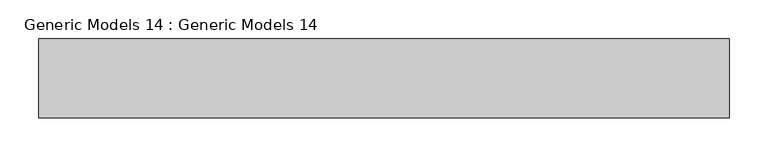
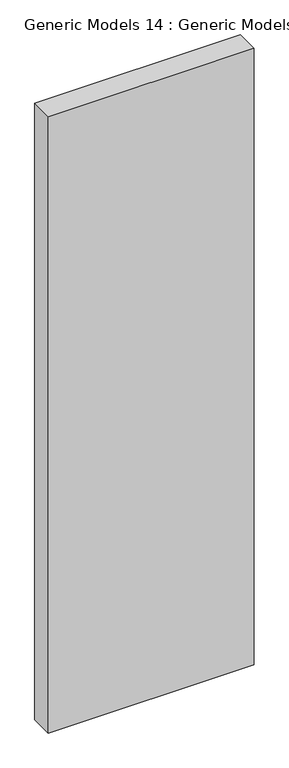
"""IFC4 building model written with IfcOpenShell, lengths in millimetres: proxy geometry, Generic Models 14 : Generic Models 14."""

from ifc_helpers import new_model, si_unit, frame, origin, place, context, project, spatial, polyline, outline, extrude, source, transform, mapped, element, save


def generic_models_14_generic_models_14_88c4d60d(model_context):
    return source(origin(), model_context, "Body", "SweptSolid", [
        extrude(outline(polyline([(1282.8673568, -11415.9323314), (1282.8673568, -11314.3323314), (2171.8673568, -11314.3323314), (2171.8673568, -11415.9323314), (1282.8673568, -11415.9323314)])), frame((0.0, 0.0, 3584.575), z_axis=(0.0, 0.0, 1.0), x_axis=(1.0, 0.0, 0.0)), (0.0, 0.0, 1.0), 2816.225),
    ])


if __name__ == "__main__":
    model = new_model("IFC4")
    model_context = context("Model", 3, world=origin())
    ifc_project = project(units=[si_unit("LENGTHUNIT", "METRE", prefix="MILLI")], contexts=[model_context])
    site = spatial("IfcSite", under=ifc_project)
    building = spatial("IfcBuilding", under=site)
    placement = place(None, origin())
    generic_models_14_generic_models_14_shape = generic_models_14_generic_models_14_88c4d60d(model_context)
    element("IfcBuildingElementProxy", 1, Name="Generic Models 14 : Generic Models 14", ObjectType="Generic Models 14 : Generic Models 14", at=placement, inside=building, context=model_context, shape_type="MappedRepresentation", body=[
        mapped(generic_models_14_generic_models_14_shape, transform((0.0, 0.0, 0.0), x_axis=(1.0, 0.0, 0.0), y_axis=(0.0, 1.0, 0.0), z_axis=(0.0, 0.0, 1.0))),
    ])
    save(model, "model.ifc")
